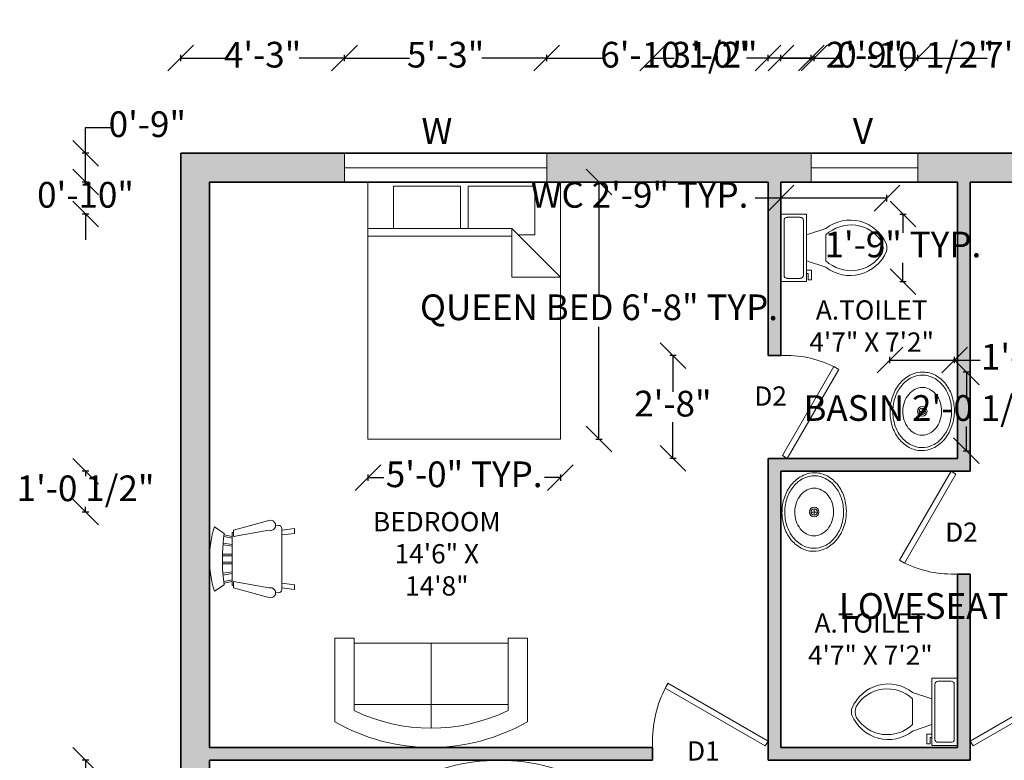
# Model space of a CAD drawing. Units: inches. Extents: x 2530 to 3100, y 543 to 1175.
# Tile 4 of 5: x 2576 to 2883, y 944 to 1175. Entities that reach past the tile are written whole.
import ezdxf

# ---------------------------------------------------------------- set-up
doc = ezdxf.new("R2010")
doc.units = ezdxf.units.IN
for name, color, linetype, lineweight in [('A-ANNO-DIMS', 2, 'Continuous', 18), ('A-ANNO-TEXT', 7, 'Continuous', 18), ('A-AREA-IDEN', 7, 'Continuous', 18), ('A-DOOR', 3, 'Continuous', 18), ('A-FLOR-FIXT', 8, 'Continuous', 18), ('A-FURN', 8, 'Continuous', 18), ('A-GLAZ', 4, 'Continuous', 18), ('A-WALL', 7, 'Continuous', 35), ('A-WALL-PATT', 30, 'Continuous', 13)]:
    doc.layers.add(name, color=color, linetype=linetype, lineweight=lineweight)
doc.styles.get("Standard").update_dxf_attribs({"font": 'arial.ttf'})
doc.dimstyles.new('ISO-25', dxfattribs={"dimtxt": 8, "dimasz": 8, "dimexe": 1, "dimexo": 1, "dimtad": 0, "dimtih": 1, "dimtoh": 1, "dimlunit": 3, "dimtxsty": 'Standard', "dimblk": 'OBLIQUE', "dimcen": 2.5, "dimadec": 0, "dimazin": 0, "dimtfac": 1, "dimtmove": 0, "dimatfit": 3, "dimfxl": 1, "dimfxlon": 1, "dimarcsym": 0})

# ---------------------------------------------------------------- blocks, each defined once
blk = doc.blocks.new('*U6')
for p, q in [((0, 0), (0, -6)), ((-32, 0), (-32, -6))]:
    blk.add_line(p, q)
blk.add_lwpolyline([(0, 0), (-27.71, 16), (-28.59, 14.48), (-0.88, -1.52)], close=True)
blk.add_arc((0, 0), 32, 150, 180)
blk = doc.blocks.new('*U4')
for p, q in [((0, 0), (0, -6)), ((36, 0), (36, -6))]:
    blk.add_line(p, q)
blk.add_lwpolyline([(0, 0), (31.18, 18), (32.05, 16.48), (0.87, -1.52)], close=True)
blk.add_arc((0, 0), 36, 0, 30)
blk = doc.blocks.new('*U5')
for p, q in [((0, 0), (0, -6)), ((-36, 0), (-36, -6))]:
    blk.add_line(p, q)
blk.add_lwpolyline([(0, 0), (-31.18, 18), (-32.05, 16.48), (-0.88, -1.52)], close=True)
blk.add_arc((0, 0), 36, 150, 180)
blk = doc.blocks.new('Toilet - top')
for p, q in [((9.5, -6), (9.5, -2)), ((-10, -8.5), (-8, -8.5)), ((-10, -9.5), (-10, -8.5)), ((-8, -8.5), (-8, -8)), ((-7, -8), (-7, -9.5)), ((-4, -8), (-6, -14)), ((4, -8), (6, -14)), ((-7, -9.5), (-10, -9.5)), ((4, -14), (-4, -14))]:
    blk.add_line(p, q)
blk.add_lwpolyline([(10.5, -8), (10.5, 0), (-10.5, 0), (-10.5, -8)], close=True)
for points in [[(-9.5, -2), (-9.5, -6)], [(8.5, -1), (-8.5, -1)], [(-8.5, -7), (8.5, -7)]]:
    blk.add_lwpolyline(points)
for centre, radius, start, end in [((-8.62, -1.88), 0.884, 81.8699, 188.1301), ((8.62, -1.88), 0.884, 351.8699, 98.1301), ((-8.62, -6.12), 0.884, 171.8699, 278.1301), ((8.62, -6.12), 0.884, 261.8699, 8.1301), ((3.52, -21.58), 12.17, 141.4691, 247.9714), ((4.2, -21.82), 11.33, 136.3677, 238.9468), ((-3.52, -21.58), 12.17, 292.0284, 38.5307), ((-4.2, -21.82), 11.33, 301.053, 43.6321), ((0, -27.88), 4, 245.7318, 294.2682), ((0, -29), 4, 254.8605, 285.1395)]:
    blk.add_arc(centre, radius, start, end)
blk = doc.blocks.new('Sink - Oval top')
for p, q in [((-1, 0), (1, 0)), ((0, 1), (0, -1))]:
    blk.add_line(p, q)
for points in [[(-12.23, 0.39, 0.117634), (-11.46, -3.36, 0.104469), (-8.88, -6.8, 0.090016), (-5.08, -9.07, 0.08192), (-0.32, -10.02, 0.08192), (4.49, -9.38, 0.090016), (8.42, -7.36, 0.104469), (11.22, -4.09, 0.117634), (12.23, -0.39, 0.117634), (11.46, 3.36, 0.104469), (8.88, 6.8, 0.090016), (5.08, 9.07, 0.08192), (0.32, 10.02, 0.08192), (-4.49, 9.38, 0.090016), (-8.42, 7.36, 0.104469), (-11.22, 4.09, 0.117634)], [(-11.29, 0.16, 0.118622), (-10.52, -3.25, 0.104678), (-8.07, -6.36, 0.089562), (-4.54, -8.37, 0.081185), (-0.13, -9.15, 0.081185), (4.3, -8.49, 0.089562), (7.89, -6.58, 0.104678), (10.42, -3.55, 0.118622), (11.29, -0.16, 0.118622), (10.52, 3.25, 0.104678), (8.07, 6.36, 0.089562), (4.54, 8.37, 0.081185), (0.13, 9.15, 0.081185), (-4.3, 8.49, 0.089562), (-7.89, 6.58, 0.104678), (-10.42, 3.55, 0.118622)], [(-7.42, 0.08, 0.118283), (-6.91, -2.17, 0.104607), (-5.29, -4.21, 0.089718), (-2.97, -5.53, 0.081436), (-0.07, -6.04, 0.081436), (2.84, -5.59, 0.089718), (5.2, -4.33, 0.104607), (6.86, -2.32, 0.118283), (7.42, -0.08, 0.118283), (6.91, 2.17, 0.104607), (5.29, 4.21, 0.089718), (2.97, 5.53, 0.081436), (0.07, 6.04, 0.081436), (-2.84, 5.59, 0.089718), (-5.2, 4.33, 0.104607), (-6.86, 2.32, 0.118283)]]:
    blk.add_lwpolyline(points, format="xyb", close=True)
for radius in [1.5, 1]:
    blk.add_circle((0, 0), radius)
blk = doc.blocks.new('Bed - Queen')
for p, q in [((0, -80.00003), (0, 0)), ((0, 0), (59.99999, 0)), ((59.99999, 0), (59.99999, -80.00003)), ((7.99999, -1.2), (28.79998, -1.2)), ((7.99999, -14.4), (7.99999, -1.2)), ((28.79998, -1.2), (28.79998, -14.4)), ((31.19999, -1.2), (51.99999, -1.2)), ((31.19999, -14.4), (31.19999, -1.2)), ((51.99999, -1.2), (51.99999, -16.4)), ((0, -14.4), (44.8, -14.4)), ((59.99999, -29.6), (44.8, -14.4)), ((44.8, -14.4), (44.8, -29.6)), ((44.8, -16.8), (0, -16.8)), ((51.99999, -16.4), (46.79936, -16.4)), ((44.8, -29.6), (59.99999, -29.6)), ((59.99999, -80.00003), (0, -80.00003))]:
    blk.add_line(p, q)
blk = doc.blocks.new('Sofa - Roundback Loveseat 5 ft.')
for p, q in [((0, -32.44198), (0, -5.99998)), ((-24, -33.99998), (-24, -11.46958)), ((24.00004, -33.99998), (24.00004, -11.46958)), ((-23.9998, -13.38178), (23.99986, -13.38178)), ((-24, -32.44198), (24.00004, -32.44198))]:
    blk.add_line(p, q)
for points in [[(-24, -33.99998), (-30, -33.99998), (-30, -7.99998)], [(30.00004, -7.99998), (30.00004, -33.99998), (24.00004, -33.99998)]]:
    blk.add_lwpolyline(points)
for centre, radius, start, end in [((0, -60.24998), 60.24998, 60.13715, 119.8628), ((0, -61.38438), 55.38444, 64.32083, 115.6792)]:
    blk.add_arc(centre, radius, start, end)
blk = doc.blocks.new('Chair - Rocking')
for p, q in [((-8, -4.5), (-10, -1.5)), ((8, -4.5), (10, -1.5)), ((-7.5, -4.5), (-7, -7)), ((-6.5, -7), (-7.02225, -4.43)), ((-4.5, -7), (-4.96674, -4.19951)), ((-4, -7), (-4.40532, -4.16272)), ((-1.5, -4.05012), (-1.5, -7)), ((-1, -7), (-1, -4.05012)), ((1, -7), (1, -4.04655)), ((1.5, -4.05012), (1.5, -7)), ((4, -7), (4.40187, -4.18694)), ((4.5, -7), (4.96761, -4.19437)), ((6.5, -7), (7, -4.4057)), ((7.5, -4.5), (7, -7)), ((-9, -7.5), (-12, -18.49999)), ((-7, -7.5), (-9, -7.5)), ((-9, -18.49999), (-7, -7.5)), ((-8.23428, -6.99939), (-8.3093, -7.47958)), ((-8.23041, -7), (8.23915, -7)), ((7, -7.5), (9, -7.5)), ((9, -18.49999), (7, -7.5)), ((8.31071, -7.48854), (8.23449, -7.00073)), ((9, -7.5), (12, -18.49999)), ((-10.36644, -20.64523), (-10.5, -21.49999)), ((10.5, -21.49999), (10.3575, -20.58798)), ((-9, -22.49999), (-9.5, -26.49999)), ((0, -22.49999), (-9.5, -22.49999)), ((-8, -26.49999), (-7.5, -22.49999)), ((0, -22.49999), (9.5, -22.49999)), ((8, -26.49999), (7.5, -22.49999)), ((9, -22.49999), (9.5, -26.49999)), ((-9.5, -26.49999), (-8, -26.49999)), ((9.5, -26.49999), (8, -26.49999))]:
    blk.add_line(p, q)
for centre, radius, start, end in [((0, -34.08333), 34.08333, 72.93847, 107.0615), ((0, -68.25004), 64.25, 93.92211, 97.15267), ((0, -68.25004), 64.25, 82.84733, 93.92211), ((-10.5, -18.99999), 1.58114, 161.5651, 18.43495), ((10.5, -18.99999), 1.58114, 161.5651, 18.43495), ((-9.5, -21.49999), 1, 180, 270), ((9.5, -21.49999), 1, 270, 0)]:
    blk.add_arc(centre, radius, start, end)
blk = doc.blocks.new('_Oblique')
at = {"color": 0, "linetype": 'ByBlock', "lineweight": -2}
blk.add_line((-0.5, -0.5), (0.5, 0.5), dxfattribs=at)
blk = doc.blocks.new('*D24')
at = {"layer": 'A-ANNO-DIMS', "color": 0, "lineweight": -2, "transparency": 16777216}
for p, q in [((2946.92, 991.41), (2938.92, 991.41)), ((2946.92, 990.41), (2946.92, 992.41)), ((3006.92, 991.41), (2946.92, 991.41)), ((3006.92, 990.41), (3006.92, 992.41))]:
    blk.add_line(p, q, dxfattribs=at)
at = {"layer": 'Defpoints', "color": 0, "transparency": 16777216}
for p in [(2946.92, 991.41), (2946.92, 982.41), (3006.92, 982.41)]:
    blk.add_point(p, dxfattribs=at)
at = {"layer": 'A-ANNO-DIMS', "color": 0, "lineweight": -2, "transparency": 16777216, "xscale": 8, "yscale": 8, "zscale": 8, "rotation": 180}
blk.add_blockref('_Oblique', (2946.92, 991.41), dxfattribs=at)
at = {"layer": 'A-ANNO-DIMS', "color": 0, "lineweight": -2, "transparency": 16777216, "xscale": 8, "yscale": 8, "zscale": 8}
blk.add_blockref('_Oblique', (3006.92, 991.41), dxfattribs=at)
at = {"layer": 'A-ANNO-DIMS', "color": 0, "transparency": 16777216, "insert": (2883.03, 991.41), "char_height": 8, "attachment_point": 5}
blk.add_mtext('LOVESEAT 5\'-0" TYP.', dxfattribs=at)
blk = doc.blocks.new('*D28')
at = {"layer": 'A-ANNO-DIMS', "color": 0, "lineweight": -2, "transparency": 16777216}
for p, q in [((2812.92, 1118.42), (2812.92, 1120.42)), ((2845.96, 1118.42), (2845.96, 1120.42)), ((2812.92, 1119.42), (2804.92, 1119.42)), ((2845.96, 1119.42), (2812.92, 1119.42))]:
    blk.add_line(p, q, dxfattribs=at)
at = {"layer": 'Defpoints', "color": 0, "transparency": 16777216}
for p in [(2812.92, 1119.42), (2812.92, 1114.46), (2845.96, 1114.46)]:
    blk.add_point(p, dxfattribs=at)
at = {"layer": 'A-ANNO-DIMS', "color": 0, "lineweight": -2, "transparency": 16777216, "xscale": 8, "yscale": 8, "zscale": 8, "rotation": 180}
blk.add_blockref('_Oblique', (2812.92, 1119.42), dxfattribs=at)
at = {"layer": 'A-ANNO-DIMS', "color": 0, "lineweight": -2, "transparency": 16777216, "xscale": 8, "yscale": 8, "zscale": 8}
blk.add_blockref('_Oblique', (2845.96, 1119.42), dxfattribs=at)
at = {"layer": 'A-ANNO-DIMS', "color": 0, "transparency": 16777216, "insert": (2768.88, 1119.42), "char_height": 8, "attachment_point": 5}
blk.add_mtext('WC 2\'-9" TYP.', dxfattribs=at)
blk = doc.blocks.new('*D29')
at = {"layer": 'A-ANNO-DIMS', "color": 0, "lineweight": -2, "transparency": 16777216}
for p, q in [((2849.92, 1114.46), (2851.92, 1114.46)), ((2850.92, 1114.46), (2850.92, 1108.67)), ((2850.92, 1093.46), (2850.92, 1099.25)), ((2849.92, 1093.46), (2851.92, 1093.46))]:
    blk.add_line(p, q, dxfattribs=at)
at = {"layer": 'Defpoints', "color": 0, "transparency": 16777216}
for p in [(2845.96, 1114.46), (2850.92, 1114.46), (2845.96, 1093.46)]:
    blk.add_point(p, dxfattribs=at)
at = {"layer": 'A-ANNO-DIMS', "color": 0, "lineweight": -2, "transparency": 16777216, "xscale": 8, "yscale": 8, "zscale": 8}
for p, rotation in [((2850.92, 1114.46), 90), ((2850.92, 1093.46), 270)]:
    blk.add_blockref('_Oblique', p, dxfattribs=dict(at, rotation=rotation))
at = {"layer": 'A-ANNO-DIMS', "color": 0, "transparency": 16777216, "insert": (2850.92, 1103.96), "char_height": 8, "attachment_point": 5}
blk.add_mtext('1\'-9" TYP.', dxfattribs=at)
blk = doc.blocks.new('*D30')
at = {"layer": 'A-ANNO-DIMS', "color": 0, "lineweight": -2, "transparency": 16777216}
for p, q in [((2869.69, 1065.33), (2871.69, 1065.33)), ((2870.69, 1065.33), (2870.69, 1057.81)), ((2870.69, 1040.78), (2870.69, 1048.29)), ((2869.69, 1040.78), (2871.69, 1040.78))]:
    blk.add_line(p, q, dxfattribs=at)
at = {"layer": 'Defpoints', "color": 0, "transparency": 16777216}
for p in [(2867.01, 1065.33), (2867.01, 1040.78), (2870.69, 1040.78)]:
    blk.add_point(p, dxfattribs=at)
at = {"layer": 'A-ANNO-DIMS', "color": 0, "lineweight": -2, "transparency": 16777216, "xscale": 8, "yscale": 8, "zscale": 8}
for p, rotation in [((2870.69, 1065.33), 90), ((2870.69, 1040.78), 270)]:
    blk.add_blockref('_Oblique', p, dxfattribs=dict(at, rotation=rotation))
at = {"layer": 'A-ANNO-DIMS', "color": 0, "transparency": 16777216, "insert": (2870.69, 1053.05), "char_height": 8, "attachment_point": 5}
blk.add_mtext('BASIN 2\'-0 1/2" TYP.', dxfattribs=at)
blk = doc.blocks.new('*D31')
at = {"layer": 'A-ANNO-DIMS', "color": 0, "lineweight": -2, "transparency": 16777216}
for p, q in [((2846.87, 1068.01), (2846.87, 1070.01)), ((2846.87, 1069.01), (2867.01, 1069.01)), ((2867.01, 1068.01), (2867.01, 1070.01)), ((2867.01, 1069.01), (2875.01, 1069.01))]:
    blk.add_line(p, q, dxfattribs=at)
at = {"layer": 'Defpoints', "color": 0, "transparency": 16777216}
for p in [(2867.01, 1069.01), (2846.87, 1065.33), (2867.01, 1065.33)]:
    blk.add_point(p, dxfattribs=at)
at = {"layer": 'A-ANNO-DIMS', "color": 0, "lineweight": -2, "transparency": 16777216, "xscale": 8, "yscale": 8, "zscale": 8, "rotation": 180}
blk.add_blockref('_Oblique', (2846.87, 1069.01), dxfattribs=at)
at = {"layer": 'A-ANNO-DIMS', "color": 0, "lineweight": -2, "transparency": 16777216, "xscale": 8, "yscale": 8, "zscale": 8}
blk.add_blockref('_Oblique', (2867.01, 1069.01), dxfattribs=at)
at = {"layer": 'A-ANNO-DIMS', "color": 0, "transparency": 16777216, "insert": (2899.64, 1069.01), "char_height": 8, "attachment_point": 5}
blk.add_mtext('1\'-8" TYP.', dxfattribs=at)
blk = doc.blocks.new('*D32')
at = {"layer": 'A-ANNO-DIMS', "color": 0, "lineweight": -2, "transparency": 16777216}
for p, q in [((2755.24, 1124.41), (2757.24, 1124.41)), ((2756.24, 1124.41), (2756.24, 1089.41)), ((2756.24, 1044.41), (2756.24, 1079.4)), ((2755.24, 1044.41), (2757.24, 1044.41))]:
    blk.add_line(p, q, dxfattribs=at)
at = {"layer": 'Defpoints', "color": 0, "transparency": 16777216}
for p in [(2744.24, 1124.41), (2756.24, 1124.41), (2744.24, 1044.41)]:
    blk.add_point(p, dxfattribs=at)
at = {"layer": 'A-ANNO-DIMS', "color": 0, "lineweight": -2, "transparency": 16777216, "xscale": 8, "yscale": 8, "zscale": 8}
for p, rotation in [((2756.24, 1124.41), 90), ((2756.24, 1044.41), 270)]:
    blk.add_blockref('_Oblique', p, dxfattribs=dict(at, rotation=rotation))
at = {"layer": 'A-ANNO-DIMS', "color": 0, "transparency": 16777216, "insert": (2756.24, 1084.41), "char_height": 8, "attachment_point": 5}
blk.add_mtext('QUEEN BED 6\'-8" TYP.', dxfattribs=at)
blk = doc.blocks.new('*D33')
at = {"layer": 'A-ANNO-DIMS', "color": 0, "lineweight": -2, "transparency": 16777216}
for p, q in [((2684.24, 1033.41), (2684.24, 1031.41)), ((2684.24, 1032.41), (2689.24, 1032.41)), ((2744.24, 1032.41), (2739.25, 1032.41)), ((2744.24, 1033.41), (2744.24, 1031.41))]:
    blk.add_line(p, q, dxfattribs=at)
at = {"layer": 'Defpoints', "color": 0, "transparency": 16777216}
for p in [(2684.24, 1044.41), (2744.24, 1044.41), (2744.24, 1032.41)]:
    blk.add_point(p, dxfattribs=at)
at = {"layer": 'A-ANNO-DIMS', "color": 0, "lineweight": -2, "transparency": 16777216, "xscale": 8, "yscale": 8, "zscale": 8, "rotation": 180}
blk.add_blockref('_Oblique', (2684.24, 1032.41), dxfattribs=at)
at = {"layer": 'A-ANNO-DIMS', "color": 0, "lineweight": -2, "transparency": 16777216, "xscale": 8, "yscale": 8, "zscale": 8}
blk.add_blockref('_Oblique', (2744.24, 1032.41), dxfattribs=at)
at = {"layer": 'A-ANNO-DIMS', "color": 0, "transparency": 16777216, "insert": (2714.24, 1032.41), "char_height": 8, "attachment_point": 5}
blk.add_mtext('5\'-0" TYP.', dxfattribs=at)
blk = doc.blocks.new('*D47')
at = {"layer": 'A-ANNO-DIMS', "color": 0, "lineweight": -2, "transparency": 16777216}
for p, q in [((2597.27, 944.41), (2595.27, 944.41)), ((2596.27, 944.41), (2596.27, 860.12)), ((2596.27, 766.41), (2596.27, 850.7)), ((2597.27, 766.41), (2595.27, 766.41))]:
    blk.add_line(p, q, dxfattribs=at)
at = {"layer": 'Defpoints', "color": 0, "transparency": 16777216}
for p in [(2596.27, 944.41), (2634.92, 944.41), (2634.92, 766.41)]:
    blk.add_point(p, dxfattribs=at)
at = {"layer": 'A-ANNO-DIMS', "color": 0, "lineweight": -2, "transparency": 16777216, "xscale": 8, "yscale": 8, "zscale": 8}
for p, rotation in [((2596.27, 944.41), 90), ((2596.27, 766.41), 270)]:
    blk.add_blockref('_Oblique', p, dxfattribs=dict(at, rotation=rotation))
at = {"layer": 'A-ANNO-DIMS', "color": 0, "transparency": 16777216, "insert": (2596.27, 855.41), "char_height": 8, "attachment_point": 5}
blk.add_mtext('14\'-10"', dxfattribs=at)
blk = doc.blocks.new('*D50')
at = {"layer": 'A-ANNO-DIMS', "color": 0, "lineweight": -2, "transparency": 16777216}
for p, q in [((2625.92, 1162.06), (2625.92, 1164.06)), ((2625.92, 1163.06), (2640.01, 1163.06)), ((2676.95, 1163.06), (2662.85, 1163.06)), ((2676.95, 1162.06), (2676.95, 1164.06))]:
    blk.add_line(p, q, dxfattribs=at)
at = {"layer": 'Defpoints', "color": 0, "transparency": 16777216}
for p in [(2676.95, 1163.06), (2625.92, 1133.41), (2676.95, 1133.41)]:
    blk.add_point(p, dxfattribs=at)
at = {"layer": 'A-ANNO-DIMS', "color": 0, "lineweight": -2, "transparency": 16777216, "xscale": 8, "yscale": 8, "zscale": 8, "rotation": 180}
blk.add_blockref('_Oblique', (2625.92, 1163.06), dxfattribs=at)
at = {"layer": 'A-ANNO-DIMS', "color": 0, "lineweight": -2, "transparency": 16777216, "xscale": 8, "yscale": 8, "zscale": 8}
blk.add_blockref('_Oblique', (2676.95, 1163.06), dxfattribs=at)
at = {"layer": 'A-ANNO-DIMS', "color": 0, "transparency": 16777216, "insert": (2651.43, 1163.06), "char_height": 8, "attachment_point": 5}
blk.add_mtext('4\'-3"', dxfattribs=at)
blk = doc.blocks.new('*D51')
at = {"layer": 'A-ANNO-DIMS', "color": 0, "lineweight": -2, "transparency": 16777216}
for p, q in [((2676.95, 1162.06), (2676.95, 1164.06)), ((2676.95, 1163.06), (2697.19, 1163.06)), ((2739.95, 1163.06), (2719.7, 1163.06)), ((2739.95, 1162.06), (2739.95, 1164.06))]:
    blk.add_line(p, q, dxfattribs=at)
at = {"layer": 'Defpoints', "color": 0, "transparency": 16777216}
for p in [(2739.95, 1163.06), (2676.95, 1133.41), (2739.95, 1133.41)]:
    blk.add_point(p, dxfattribs=at)
at = {"layer": 'A-ANNO-DIMS', "color": 0, "lineweight": -2, "transparency": 16777216, "xscale": 8, "yscale": 8, "zscale": 8, "rotation": 180}
blk.add_blockref('_Oblique', (2676.95, 1163.06), dxfattribs=at)
at = {"layer": 'A-ANNO-DIMS', "color": 0, "lineweight": -2, "transparency": 16777216, "xscale": 8, "yscale": 8, "zscale": 8}
blk.add_blockref('_Oblique', (2739.95, 1163.06), dxfattribs=at)
at = {"layer": 'A-ANNO-DIMS', "color": 0, "transparency": 16777216, "insert": (2708.45, 1163.06), "char_height": 8, "attachment_point": 5}
blk.add_mtext('5\'-3"', dxfattribs=at)
blk = doc.blocks.new('*D52')
at = {"layer": 'A-ANNO-DIMS', "color": 0, "lineweight": -2, "transparency": 16777216}
for p, q in [((2739.95, 1162.06), (2739.95, 1164.06)), ((2739.95, 1163.06), (2757.44, 1163.06)), ((2822.35, 1163.06), (2804.85, 1163.06)), ((2822.35, 1162.06), (2822.35, 1164.06))]:
    blk.add_line(p, q, dxfattribs=at)
at = {"layer": 'Defpoints', "color": 0, "transparency": 16777216}
for p in [(2822.35, 1163.06), (2739.95, 1133.41), (2822.35, 1133.41)]:
    blk.add_point(p, dxfattribs=at)
at = {"layer": 'A-ANNO-DIMS', "color": 0, "lineweight": -2, "transparency": 16777216, "xscale": 8, "yscale": 8, "zscale": 8, "rotation": 180}
blk.add_blockref('_Oblique', (2739.95, 1163.06), dxfattribs=at)
at = {"layer": 'A-ANNO-DIMS', "color": 0, "lineweight": -2, "transparency": 16777216, "xscale": 8, "yscale": 8, "zscale": 8}
blk.add_blockref('_Oblique', (2822.35, 1163.06), dxfattribs=at)
at = {"layer": 'A-ANNO-DIMS', "color": 0, "transparency": 16777216, "insert": (2781.15, 1163.06), "char_height": 8, "attachment_point": 5}
blk.add_mtext('6\'-10 1/2"', dxfattribs=at)
blk = doc.blocks.new('*D53')
at = {"layer": 'A-ANNO-DIMS', "color": 0, "lineweight": -2, "transparency": 16777216}
for p, q in [((2822.35, 1162.06), (2822.35, 1164.06)), ((2822.35, 1163.06), (2827.63, 1163.06)), ((2855.56, 1163.06), (2850.28, 1163.06)), ((2855.56, 1162.06), (2855.56, 1164.06))]:
    blk.add_line(p, q, dxfattribs=at)
at = {"layer": 'Defpoints', "color": 0, "transparency": 16777216}
for p in [(2855.56, 1163.06), (2822.35, 1133.41), (2855.56, 1133.41)]:
    blk.add_point(p, dxfattribs=at)
at = {"layer": 'A-ANNO-DIMS', "color": 0, "lineweight": -2, "transparency": 16777216, "xscale": 8, "yscale": 8, "zscale": 8, "rotation": 180}
blk.add_blockref('_Oblique', (2822.35, 1163.06), dxfattribs=at)
at = {"layer": 'A-ANNO-DIMS', "color": 0, "lineweight": -2, "transparency": 16777216, "xscale": 8, "yscale": 8, "zscale": 8}
blk.add_blockref('_Oblique', (2855.56, 1163.06), dxfattribs=at)
at = {"layer": 'A-ANNO-DIMS', "color": 0, "transparency": 16777216, "insert": (2838.95, 1163.06), "char_height": 8, "attachment_point": 5}
blk.add_mtext('2\'-9"', dxfattribs=at)
blk = doc.blocks.new('*D54')
at = {"layer": 'A-ANNO-DIMS', "color": 0, "lineweight": -2, "transparency": 16777216}
for p, q in [((2855.56, 1162.06), (2855.56, 1164.06)), ((2855.56, 1163.06), (2877.19, 1163.06)), ((2939.91, 1163.06), (2918.28, 1163.06)), ((2939.91, 1162.06), (2939.91, 1164.06))]:
    blk.add_line(p, q, dxfattribs=at)
at = {"layer": 'Defpoints', "color": 0, "transparency": 16777216}
for p in [(2939.91, 1163.06), (2855.56, 1133.41), (2939.91, 1133.41)]:
    blk.add_point(p, dxfattribs=at)
at = {"layer": 'A-ANNO-DIMS', "color": 0, "lineweight": -2, "transparency": 16777216, "xscale": 8, "yscale": 8, "zscale": 8, "rotation": 180}
blk.add_blockref('_Oblique', (2855.56, 1163.06), dxfattribs=at)
at = {"layer": 'A-ANNO-DIMS', "color": 0, "lineweight": -2, "transparency": 16777216, "xscale": 8, "yscale": 8, "zscale": 8}
blk.add_blockref('_Oblique', (2939.91, 1163.06), dxfattribs=at)
at = {"layer": 'A-ANNO-DIMS', "color": 0, "transparency": 16777216, "insert": (2897.74, 1163.06), "char_height": 8, "attachment_point": 5}
blk.add_mtext('7\'-0 1/2"', dxfattribs=at)
blk = doc.blocks.new('*D62')
at = {"layer": 'A-ANNO-DIMS', "color": 0, "lineweight": -2, "transparency": 16777216}
for p, q in [((2772.92, 1162.06), (2772.92, 1164.06)), ((2772.92, 1163.06), (2779.66, 1163.06)), ((2808.92, 1163.06), (2802.17, 1163.06)), ((2808.92, 1162.06), (2808.92, 1164.06))]:
    blk.add_line(p, q, dxfattribs=at)
at = {"layer": 'Defpoints', "color": 0, "transparency": 16777216}
for p in [(2808.92, 1163.06), (2772.92, 948.41), (2808.92, 948.66)]:
    blk.add_point(p, dxfattribs=at)
at = {"layer": 'A-ANNO-DIMS', "color": 0, "lineweight": -2, "transparency": 16777216, "xscale": 8, "yscale": 8, "zscale": 8, "rotation": 180}
blk.add_blockref('_Oblique', (2772.92, 1163.06), dxfattribs=at)
at = {"layer": 'A-ANNO-DIMS', "color": 0, "lineweight": -2, "transparency": 16777216, "xscale": 8, "yscale": 8, "zscale": 8}
blk.add_blockref('_Oblique', (2808.92, 1163.06), dxfattribs=at)
at = {"layer": 'A-ANNO-DIMS', "color": 0, "transparency": 16777216, "insert": (2790.92, 1163.06), "char_height": 8, "attachment_point": 5}
blk.add_mtext('3\'-0"', dxfattribs=at)
blk = doc.blocks.new('*D63')
at = {"layer": 'A-ANNO-DIMS', "color": 0, "lineweight": -2, "transparency": 16777216}
for p, q in [((2780.27, 1070.41), (2778.27, 1070.41)), ((2779.27, 1070.41), (2779.27, 1059.12)), ((2779.27, 1038.41), (2779.27, 1049.7)), ((2780.27, 1038.41), (2778.27, 1038.41))]:
    blk.add_line(p, q, dxfattribs=at)
at = {"layer": 'Defpoints', "color": 0, "transparency": 16777216}
for p in [(2779.27, 1070.41), (2808.92, 1070.41), (2808.92, 1038.41)]:
    blk.add_point(p, dxfattribs=at)
at = {"layer": 'A-ANNO-DIMS', "color": 0, "lineweight": -2, "transparency": 16777216, "xscale": 8, "yscale": 8, "zscale": 8}
for p, rotation in [((2779.27, 1070.41), 90), ((2779.27, 1038.41), 270)]:
    blk.add_blockref('_Oblique', p, dxfattribs=dict(at, rotation=rotation))
at = {"layer": 'A-ANNO-DIMS', "color": 0, "transparency": 16777216, "insert": (2779.27, 1054.41), "char_height": 8, "attachment_point": 5}
blk.add_mtext('2\'-8"', dxfattribs=at)
blk = doc.blocks.new('*D71')
at = {"layer": 'A-ANNO-DIMS', "color": 0, "lineweight": -2, "transparency": 16777216}
for p, q in [((2596.27, 1133.41), (2596.27, 1141.41)), ((2596.27, 1141.41), (2604.27, 1141.41)), ((2597.27, 1133.41), (2595.27, 1133.41)), ((2596.27, 1124.41), (2596.27, 1133.41)), ((2597.27, 1124.41), (2595.27, 1124.41))]:
    blk.add_line(p, q, dxfattribs=at)
at = {"layer": 'Defpoints', "color": 0, "transparency": 16777216}
for p in [(2596.27, 1133.41), (2625.92, 1133.41), (2634.92, 1124.41)]:
    blk.add_point(p, dxfattribs=at)
at = {"layer": 'A-ANNO-DIMS', "color": 0, "lineweight": -2, "transparency": 16777216, "xscale": 8, "yscale": 8, "zscale": 8}
for p, rotation in [((2596.27, 1133.41), 90), ((2596.27, 1124.41), 270)]:
    blk.add_blockref('_Oblique', p, dxfattribs=dict(at, rotation=rotation))
at = {"layer": 'A-ANNO-DIMS', "color": 0, "transparency": 16777216, "insert": (2615.53, 1141.41), "char_height": 8, "attachment_point": 5}
blk.add_mtext('0\'-9"', dxfattribs=at)
blk = doc.blocks.new('*D79')
at = {"layer": 'A-ANNO-DIMS', "color": 0, "lineweight": -2, "transparency": 16777216}
for p, q in [((2596.27, 1124.41), (2596.27, 1132.41)), ((2597.27, 1124.41), (2595.27, 1124.41)), ((2596.27, 1124.41), (2596.27, 1124.14)), ((2597.27, 1114.46), (2595.27, 1114.46)), ((2596.27, 1114.46), (2596.27, 1114.72)), ((2596.27, 1114.46), (2596.27, 1106.46))]:
    blk.add_line(p, q, dxfattribs=at)
at = {"layer": 'Defpoints', "color": 0, "transparency": 16777216}
for p in [(2596.27, 1124.41), (2812.92, 1124.41), (2812.92, 1114.46)]:
    blk.add_point(p, dxfattribs=at)
at = {"layer": 'A-ANNO-DIMS', "color": 0, "lineweight": -2, "transparency": 16777216, "xscale": 8, "yscale": 8, "zscale": 8}
for p, rotation in [((2596.27, 1124.41), 270), ((2596.27, 1114.46), 90)]:
    blk.add_blockref('_Oblique', p, dxfattribs=dict(at, rotation=rotation))
at = {"layer": 'A-ANNO-DIMS', "color": 0, "transparency": 16777216, "insert": (2596.27, 1119.43), "char_height": 8, "attachment_point": 5}
blk.add_mtext('0\'-10"', dxfattribs=at)
blk = doc.blocks.new('*D80')
at = {"layer": 'A-ANNO-DIMS', "color": 0, "lineweight": -2, "transparency": 16777216}
for p, q in [((2812.92, 1162.06), (2812.92, 1164.06)), ((2812.92, 1163.06), (2823.28, 1163.06)), ((2823.28, 1162.06), (2823.28, 1164.06)), ((2823.28, 1163.06), (2831.28, 1163.06))]:
    blk.add_line(p, q, dxfattribs=at)
at = {"layer": 'Defpoints', "color": 0, "transparency": 16777216}
for p in [(2823.28, 1163.06), (2812.92, 1034.41), (2823.28, 1021.7)]:
    blk.add_point(p, dxfattribs=at)
at = {"layer": 'A-ANNO-DIMS', "color": 0, "lineweight": -2, "transparency": 16777216, "xscale": 8, "yscale": 8, "zscale": 8, "rotation": 180}
blk.add_blockref('_Oblique', (2812.92, 1163.06), dxfattribs=at)
at = {"layer": 'A-ANNO-DIMS', "color": 0, "lineweight": -2, "transparency": 16777216, "xscale": 8, "yscale": 8, "zscale": 8}
blk.add_blockref('_Oblique', (2823.28, 1163.06), dxfattribs=at)
at = {"layer": 'A-ANNO-DIMS', "color": 0, "transparency": 16777216, "insert": (2854.97, 1163.06), "char_height": 8, "attachment_point": 5}
blk.add_mtext('0\'-10 1/2"', dxfattribs=at)
blk = doc.blocks.new('*D81')
at = {"layer": 'A-ANNO-DIMS', "color": 0, "lineweight": -2, "transparency": 16777216}
for p, q in [((2597.27, 1034.41), (2595.27, 1034.41)), ((2596.27, 1034.41), (2596.27, 1032.82)), ((2597.27, 1021.7), (2595.27, 1021.7)), ((2596.27, 1021.7), (2596.27, 1023.29))]:
    blk.add_line(p, q, dxfattribs=at)
at = {"layer": 'Defpoints', "color": 0, "transparency": 16777216}
for p in [(2812.92, 1034.41), (2596.27, 1021.7), (2823.28, 1021.7)]:
    blk.add_point(p, dxfattribs=at)
at = {"layer": 'A-ANNO-DIMS', "color": 0, "lineweight": -2, "transparency": 16777216, "xscale": 8, "yscale": 8, "zscale": 8}
for p, rotation in [((2596.27, 1034.41), 90), ((2596.27, 1021.7), 270)]:
    blk.add_blockref('_Oblique', p, dxfattribs=dict(at, rotation=rotation))
at = {"layer": 'A-ANNO-DIMS', "color": 0, "transparency": 16777216, "insert": (2596.27, 1028.05), "char_height": 8, "attachment_point": 5}
blk.add_mtext('1\'-0 1/2"', dxfattribs=at)

msp = doc.modelspace()

# ---------------------------------------------------------------- hatches: boundary and pattern name
at = {"layer": 'A-WALL-PATT'}
h = msp.add_hatch(color=256, dxfattribs=at)
h.dxf.hatch_style = 1
h.paths.add_polyline_path([(2676.945, 1133.407), (2625.918, 1133.407), (2625.918, 584.407), (2673.585, 584.407), (2673.585, 593.407), (2634.918, 593.407), (2634.918, 757.407), (2717.918, 757.407), (2717.918, 766.407), (2634.918, 766.407), (2634.918, 944.407), (2772.918, 944.407), (2772.918, 948.407), (2634.918, 948.407), (2634.918, 1124.407), (2676.945, 1124.407)])
h.paths.add_polyline_path([(2822.346, 1133.407), (2739.946, 1133.407), (2739.946, 1124.407), (2808.918, 1124.407), (2808.918, 1070.407), (2812.918, 1070.407), (2812.918, 1124.407), (2822.346, 1124.407)])
h.paths.add_polyline_path([(2939.91, 1133.407), (2855.561, 1133.407), (2855.561, 1124.407), (2867.918, 1124.407), (2867.918, 1038.407), (2808.918, 1038.407), (2808.918, 944.407), (2871.918, 944.407), (2871.918, 1002.407), (2867.918, 1002.407), (2867.918, 948.407), (2812.918, 948.407), (2812.918, 1034.407), (2871.918, 1034.407), (2871.918, 1124.407), (2939.91, 1124.407)])
h.paths.add_polyline_path([(3054.918, 1133.407), (2997.969, 1133.407), (2997.969, 1124.407), (3045.918, 1124.407), (3045.918, 948.407), (2907.918, 948.407), (2907.918, 928.407), (2911.918, 928.407), (2911.918, 944.407), (2952.418, 944.407), (2952.418, 872.407), (2911.918, 872.407), (2911.918, 888.407), (2907.918, 888.407), (2907.918, 861.407), (2911.918, 861.407), (2911.918, 867.407), (2956.918, 867.407), (2956.918, 944.407), (3045.918, 944.407), (3045.918, 872.407), (2988.918, 872.407), (2988.918, 867.407), (3045.918, 867.407), (3045.918, 766.407), (2986.918, 766.407), (2986.918, 757.407), (3045.918, 757.407), (3045.918, 593.407), (2906.263, 593.407), (2906.263, 584.407), (3054.918, 584.407)])
h.paths.add_polyline_path([(2780.418, 593.407), (2762.418, 593.407), (2762.418, 693.907), (2757.918, 693.907), (2757.918, 593.407), (2719.35, 593.407), (2719.35, 584.407), (2780.418, 584.407)])
h.paths.add_polyline_path([(2846.356, 593.407), (2826.918, 593.407), (2826.918, 757.407), (2826.918, 766.407), (2822.418, 766.407), (2822.418, 693.907), (2794.418, 693.907), (2794.418, 689.407), (2822.418, 689.407), (2822.418, 593.407), (2804.418, 593.407), (2804.418, 584.407), (2846.356, 584.407)])
h.paths.add_polyline_path([(2938.918, 766.407), (2911.918, 766.407), (2911.918, 829.407), (2907.918, 829.407), (2907.918, 766.407), (2886.918, 766.407), (2886.918, 757.407), (2938.918, 757.407)])
h.paths.add_polyline_path([(2822.418, 766.407), (2757.918, 766.407), (2757.918, 757.407), (2757.918, 721.407), (2762.418, 721.407), (2762.418, 757.407), (2822.418, 757.407)])

# ---------------------------------------------------------------- linework, layer by layer
at = {"layer": 'A-GLAZ'}
for p, q in [((2676.945, 1124.407), (2676.945, 1133.407)), ((2739.946, 1124.407), (2739.946, 1133.407)), ((2822.346, 1124.407), (2822.346, 1133.407)), ((2855.561, 1124.407), (2855.561, 1133.407)), ((2676.945, 1128.907), (2739.946, 1128.907)), ((2855.561, 1128.907), (2822.346, 1128.907))]:
    msp.add_line(p, q, dxfattribs=at)
at = {"layer": 'A-WALL'}
for p, q in [((3054.918, 1133.407), (2625.918, 1133.407)), ((2625.918, 1133.407), (2625.918, 584.407)), ((2634.918, 1124.407), (2634.918, 948.407)), ((2808.918, 1124.407), (2634.918, 1124.407)), ((2808.918, 1124.407), (2808.918, 1070.407)), ((2812.918, 1124.407), (2812.918, 1070.407)), ((2867.918, 1124.407), (2812.918, 1124.407)), ((2867.918, 1038.407), (2867.918, 1124.407)), ((3045.918, 1124.407), (2871.918, 1124.407)), ((2871.918, 1034.407), (2871.918, 1124.407)), ((2808.918, 1070.407), (2812.918, 1070.407)), ((2867.918, 1038.407), (2808.918, 1038.407)), ((2808.918, 1038.407), (2808.918, 944.407)), ((2871.918, 1034.407), (2812.918, 1034.407)), ((2812.918, 1034.407), (2812.918, 948.407)), ((2867.918, 948.407), (2867.918, 1002.407)), ((2867.918, 1002.407), (2871.918, 1002.407)), ((2871.918, 944.407), (2871.918, 1002.407)), ((2772.918, 948.407), (2634.918, 948.407)), ((2772.918, 944.407), (2772.918, 948.407)), ((2867.918, 948.407), (2812.918, 948.407)), ((2634.918, 944.407), (2634.918, 766.407)), ((2772.918, 944.407), (2634.918, 944.407)), ((2871.918, 944.407), (2808.918, 944.407))]:
    msp.add_line(p, q, dxfattribs=at)

# ---------------------------------------------------------------- block references
at = {"layer": 'A-DOOR'}
for p, rotation in [((2814.918, 1038.407), 270), ((2865.918, 1034.407), 90)]:
    msp.add_blockref('*U6', p, dxfattribs=dict(at, rotation=rotation))
for name, p in [('*U5', (2808.918, 950.407)), ('*U4', (2871.918, 950.407))]:
    msp.add_blockref(name, p, dxfattribs=at)
at = {"layer": 'A-FLOR-FIXT'}
for name, p, rotation in [('Toilet - top', (2812.918, 1103.961), 90), ('Sink - Oval top', (2856.943, 1053.053), 270), ('Sink - Oval top', (2823.28, 1021.702), 270)]:
    msp.add_blockref(name, p, dxfattribs=dict(at, rotation=rotation))
at = {"layer": 'A-FLOR-FIXT', "xscale": -1, "rotation": 270}
msp.add_blockref('Toilet - top', (2867.918, 959.519), dxfattribs=at)
at = {"layer": 'A-FURN'}
for name, p in [('Bed - Queen', (2684.243, 1124.407)), ('Sofa - Roundback Loveseat 5 ft.', (2725.07, 944.407))]:
    msp.add_blockref(name, p, dxfattribs=at)
at = {"layer": 'A-FURN', "rotation": 89.99999999999999}
msp.add_blockref('Chair - Rocking', (2634.917, 1007.054), dxfattribs=at)
at = {"layer": 'A-FURN', "xscale": -1, "rotation": 180}
msp.add_blockref('Sofa - Roundback Loveseat 5 ft.', (2703.918, 948.407), dxfattribs=at)

# ---------------------------------------------------------------- texts
at = {"layer": 'A-ANNO-TEXT', "attachment_point": 1}
for s, insert, char_height in [('\\pxqc;W', (2696.495, 1144.337), 8), ('\\pxqc;V', (2829.22, 1144.337), 8), ('\\pxqc;D2', (2800.462, 1060.807), 6), ('\\pxqc;D2', (2859.935, 1018.428), 6), ('\\pxqc;D1', (2779.529, 950.326), 6)]:
    msp.add_mtext_dynamic_manual_height_columns(s, width=18.48176, gutter_width=12.5, heights=[0], dxfattribs=dict(at, insert=insert, char_height=char_height))
at = {"layer": 'A-AREA-IDEN', "char_height": 6, "attachment_point": 1}
for s, insert in [('\\pxqc;A.TOILET\\P4\'7" X 7\'2"', (2817.374, 1087.612)), ('\\pxqc;BEDROOM\\P14\'6" X 14\'8"', (2681.89, 1021.708)), ('\\pxqc;A.TOILET\\P4\'7" X 7\'2"', (2816.947, 990.148))]:
    msp.add_mtext_dynamic_manual_height_columns(s, width=47.65744, gutter_width=12.5, heights=[0], dxfattribs=dict(at, insert=insert))

# ---------------------------------------------------------------- dimensions: what is measured, and where the dimension line sits
at = {"layer": 'A-ANNO-DIMS'}
for base, p1, p2, picture, middle in [((2822.346, 1163.057), (2739.946, 1133.407), (2822.346, 1133.407), '*D52', (2781.146, 1163.057)), ((2823.28, 1163.057), (2812.918, 1034.407), (2823.28, 1021.702), '*D80', (2854.966, 1163.057)), ((2939.91, 1163.057), (2855.561, 1133.407), (2939.91, 1133.407), '*D54', (2897.736, 1163.057)), ((2676.945, 1163.057), (2625.918, 1133.407), (2676.945, 1133.407), '*D50', (2651.431, 1163.057)), ((2739.946, 1163.057), (2676.945, 1133.407), (2739.946, 1133.407), '*D51', (2708.446, 1163.057)), ((2808.918, 1163.057), (2772.918, 948.407), (2808.918, 948.657), '*D62', (2790.918, 1163.057)), ((2855.561, 1163.057), (2822.346, 1133.407), (2855.561, 1133.407), '*D53', (2838.954, 1163.057))]:
    dim = msp.add_linear_dim(base=base, p1=p1, p2=p2, dimstyle='ISO-25', override={"dimdec": 1, "dimlfac": 1, "dimrnd": 0, "dimzin": 1, "dimdsep": 46, "dimlunit": 4, "dimfrac": 2}, dxfattribs=at)
    dim.commit()
    dim.dimension.update_dxf_attribs({"geometry": picture, "text_midpoint": middle})
for base, p1, p2, picture, middle in [((2596.268, 1133.407), (2634.918, 1124.407), (2625.918, 1133.407), '*D71', (2615.526, 1141.407)), ((2596.268, 1124.407), (2812.918, 1114.461), (2812.918, 1124.407), '*D79', (2596.268, 1119.434)), ((2779.268, 1070.407), (2808.918, 1038.407), (2808.918, 1070.407), '*D63', (2779.268, 1054.407)), ((2596.268, 1021.702), (2812.918, 1034.407), (2823.28, 1021.702), '*D81', (2596.268, 1028.054)), ((2596.268, 944.407), (2634.918, 766.407), (2634.918, 944.407), '*D47', (2596.268, 855.407))]:
    dim = msp.add_linear_dim(base=base, p1=p1, p2=p2, angle=90, dimstyle='ISO-25', override={"dimdec": 1, "dimlfac": 1, "dimrnd": 0, "dimzin": 1, "dimdsep": 46, "dimlunit": 4, "dimfrac": 2}, dxfattribs=at)
    dim.commit()
    dim.dimension.update_dxf_attribs({"geometry": picture, "text_midpoint": middle})
for base, p1, p2, angle, text, picture, middle in [((2812.918, 1119.418), (2845.964, 1114.461), (2812.918, 1114.461), 180, 'WC <> TYP.', '*D28', (2768.885, 1119.418)), ((2756.243, 1124.407), (2744.243, 1044.407), (2744.243, 1124.407), 90, 'QUEEN BED <> TYP.', '*D32', (2756.243, 1084.407)), ((2850.921, 1114.461), (2845.964, 1093.461), (2845.964, 1114.461), 90, '<> TYP.', '*D29', (2850.921, 1103.961)), ((2870.6936, 1040.7776), (2867.011, 1065.3285), (2867.011, 1040.7776), 270, 'BASIN <> TYP.', '*D30', (2870.6936, 1053.053)), ((2946.917, 991.407), (3006.918, 982.407), (2946.917, 982.407), 180, 'LOVESEAT <> TYP.', '*D24', (2883.032, 991.407))]:
    dim = msp.add_linear_dim(base=base, p1=p1, p2=p2, angle=angle, text=text, dimstyle='ISO-25', override={"dimdec": 1, "dimlfac": 1, "dimrnd": 0, "dimzin": 1, "dimdsep": 46, "dimlunit": 4, "dimfrac": 2}, dxfattribs=at)
    dim.commit()
    dim.dimension.update_dxf_attribs({"geometry": picture, "text_midpoint": middle})
for base, p1, p2, picture, middle in [((2867.011, 1069.011), (2846.874, 1065.328), (2867.011, 1065.328), '*D31', (2899.641, 1069.011)), ((2744.243, 1032.407), (2684.243, 1044.407), (2744.243, 1044.407), '*D33', (2714.243, 1032.407))]:
    dim = msp.add_linear_dim(base=base, p1=p1, p2=p2, text='<> TYP.', dimstyle='ISO-25', override={"dimdec": 1, "dimlfac": 1, "dimrnd": 0, "dimzin": 1, "dimdsep": 46, "dimlunit": 4, "dimfrac": 2}, dxfattribs=at)
    dim.commit()
    dim.dimension.update_dxf_attribs({"geometry": picture, "text_midpoint": middle})

doc.saveas('drawing.dxf')
